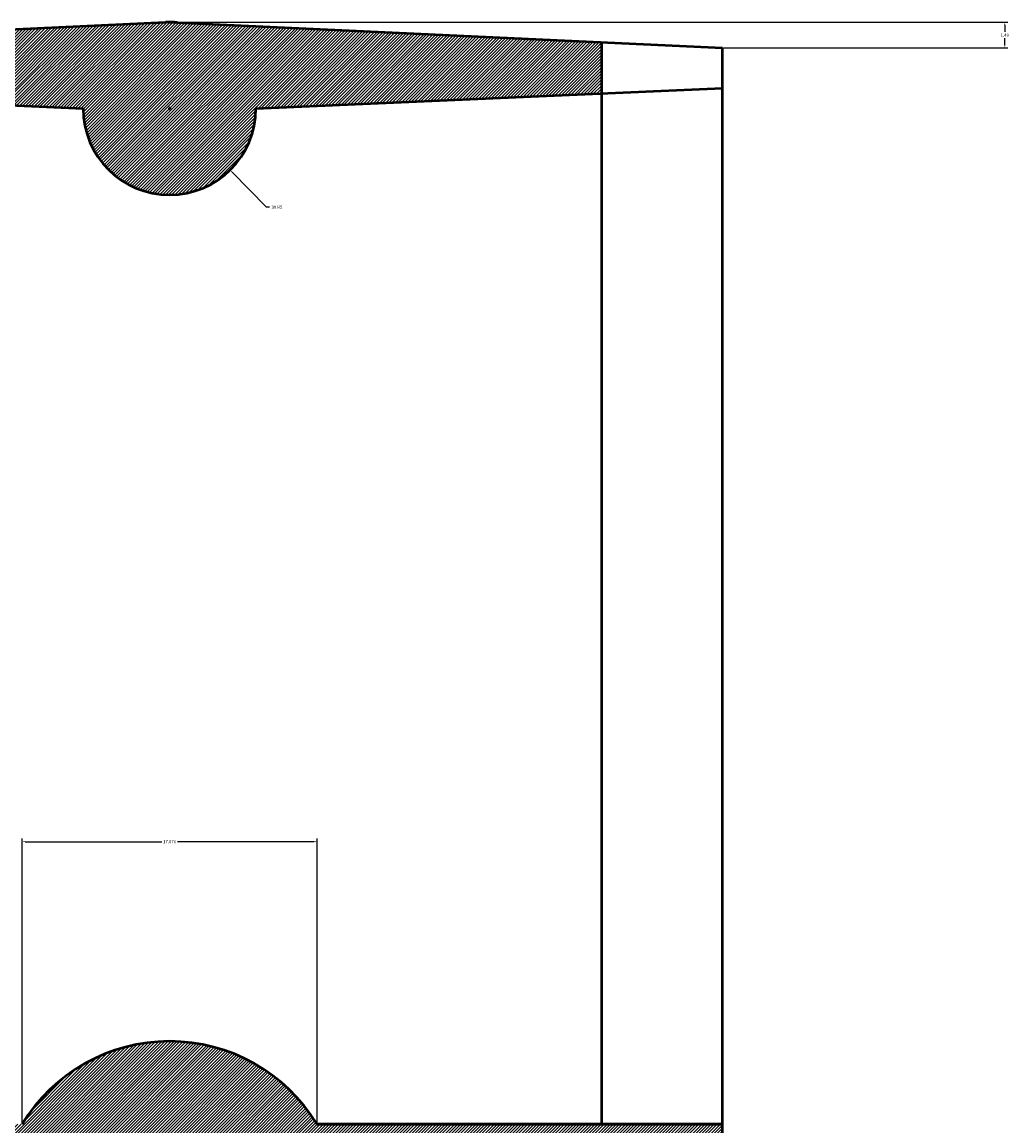
# Model space of a CAD drawing. Units: inches. Extents: x -99 to 284, y -92 to 134.
# Tile 16 of 16: x 227 to 284, y 39 to 103. Entities that reach past the tile are written whole.
import ezdxf

# ---------------------------------------------------------------- set-up
doc = ezdxf.new("R2010")
doc.units = ezdxf.units.IN
doc.header["$MEASUREMENT"] = 0
for name, color, linetype, lineweight in [('M-DIMS', 2, 'Continuous', 18), ('M-HATC', 8, 'Continuous', 18), ('M-OUTL', 7, 'Continuous', 50)]:
    doc.layers.add(name, color=color, linetype=linetype, lineweight=lineweight)
doc.styles.get("Standard").update_dxf_attribs({"font": 'arial.ttf'})
doc.dimstyles.get("Standard").update_dxf_attribs({"dimtxt": 0.18, "dimasz": 0.18, "dimexe": 0.18, "dimexo": 0.0625, "dimgap": 0.09, "dimtad": 0, "dimtih": 1, "dimtoh": 1, "dimdec": 4, "dimzin": 0, "dimdsep": 46, "dimtxsty": 'Standard', "dimcen": 0.09, "dimadec": 0, "dimazin": 0, "dimtfac": 1, "dimtdec": 4, "dimtofl": 0, "dimtmove": 0, "dimatfit": 3, "dimfxl": 1, "dimtolj": 1, "dimtzin": 0, "dimarcsym": 0})

# ---------------------------------------------------------------- blocks, each defined once
blk = doc.blocks.new('*D6')
at = {"layer": 'Defpoints', "color": 0, "transparency": 16777216}
for p in [(244.029, 55.296), (226.953, 38.946), (244.029, 38.946)]:
    blk.add_point(p, dxfattribs=at)
at = {"layer": 'M-DIMS', "color": 0, "lineweight": -2, "transparency": 16777216}
for p, q in [((226.953, 39.008), (226.953, 55.476)), ((227.133, 55.296), (235.036, 55.296)), ((243.849, 55.296), (235.946, 55.296)), ((244.029, 39.008), (244.029, 55.476))]:
    blk.add_line(p, q, dxfattribs=at)
at = {"layer": 'M-DIMS', "color": 0, "transparency": 16777216}
for points in [[(227.133, 55.326), (227.133, 55.266), (226.953, 55.296)], [(243.849, 55.326), (243.849, 55.266), (244.029, 55.296)]]:
    blk.add_solid(points, dxfattribs=at)
at = {"layer": 'M-DIMS', "color": 0, "transparency": 16777216, "insert": (235.491, 55.296), "char_height": 0.18, "attachment_point": 5}
blk.add_mtext('\\A1;17.076', dxfattribs=at)
blk = doc.blocks.new('*D11')
at = {"layer": 'Defpoints', "color": 0, "transparency": 16777216}
for p in [(235.608, 102.738), (283.841, 102.738), (267.491, 101.245)]:
    blk.add_point(p, dxfattribs=at)
at = {"layer": 'M-DIMS', "color": 0, "lineweight": -2, "transparency": 16777216}
for p, q in [((235.67, 102.738), (284.021, 102.738)), ((283.841, 102.558), (283.841, 102.173)), ((283.841, 101.425), (283.841, 101.81)), ((267.554, 101.245), (284.021, 101.245))]:
    blk.add_line(p, q, dxfattribs=at)
at = {"layer": 'M-DIMS', "color": 0, "transparency": 16777216}
for points in [[(283.811, 102.558), (283.871, 102.558), (283.841, 102.738)], [(283.811, 101.425), (283.871, 101.425), (283.841, 101.245)]]:
    blk.add_solid(points, dxfattribs=at)
at = {"layer": 'M-DIMS', "color": 0, "transparency": 16777216, "insert": (283.841, 101.992), "char_height": 0.18, "attachment_point": 5}
blk.add_mtext('\\A1;1.49', dxfattribs=at)
blk = doc.blocks.new('*D23')
at = {"layer": 'Defpoints', "color": 0, "transparency": 16777216}
for p in [(235.491, 97.74), (238.996, 94.174)]:
    blk.add_point(p, dxfattribs=at)
at = {"layer": 'M-DIMS', "color": 0, "lineweight": -2, "transparency": 16777216}
for p, q in [((235.491, 97.65), (235.491, 97.83)), ((235.401, 97.74), (235.581, 97.74)), ((241.099, 92.034), (239.122, 94.045)), ((241.279, 92.034), (241.099, 92.034))]:
    blk.add_line(p, q, dxfattribs=at)
at = {"layer": 'M-DIMS', "color": 0, "transparency": 16777216}
blk.add_solid([(239.144, 94.066), (239.101, 94.024), (238.996, 94.174)], dxfattribs=at)
at = {"layer": 'M-DIMS', "color": 0, "transparency": 16777216, "insert": (241.708, 92.034), "char_height": 0.18, "attachment_point": 5}
blk.add_mtext('\\A1;3X R5', dxfattribs=at)

msp = doc.modelspace()

# ---------------------------------------------------------------- hatches: boundary and pattern name
at = {"layer": 'M-HATC'}
h = msp.add_hatch(dxfattribs=at)
h.set_pattern_fill('ANSI31', color=256)
h.set_pattern_definition([(45, (-295.18303, 0), (-0.088388348, 0.088388348), [])])
h.paths.add_polyline_path([(235.9574, 102.7178), (260.4913, 101.5718), (260.4913, 98.6088), (240.4913, 97.7396, -1), (230.4913, 97.7396), (210.4913, 98.6088), (210.4913, 101.573), (235.4326, 102.7424), (235.4913, 102.7396, -0.0233428)])
h.paths.add_polyline_path([(226.9535, 38.946), (203.4913, 38.946), (203.4913, 30.5521), (267.4913, 30.5521), (267.4913, 38.946), (244.0291, 38.946, 0.5614625)])
h.paths.add_polyline_path([(267.4913, 30.5521), (203.4913, 30.5521), (203.4913, 28.5521), (267.4913, 28.5521)])
h.paths.add_polyline_path([(244.0291, -11.4667), (267.4913, -11.4667), (267.4913, -0.9688), (203.4913, -0.9688), (203.4913, -11.4667), (226.9535, -11.4667), (226.9535, -60.8393, -0.294228), (221.0875, -69.9448), (249.6222, -69.8159, -0.2860474), (244.0291, -60.8393)])
h.paths.add_polyline_path([(267.4913, -71.4338), (253.5949, -70.8299, -0.1036016), (249.6222, -69.8159), (221.0875, -69.9448, -0.095981), (217.3877, -70.8299), (203.4913, -71.4338), (203.4913, -73.7656), (235.2571, -75.2549, 0.0117126), (235.4913, -75.2604), (267.4913, -73.7656)])

# ---------------------------------------------------------------- linework, layer by layer
at = {"layer": 'M-OUTL'}
for p, q in [((203.4913, 101.2449), (235.2571, 102.7341)), ((235.4913, 102.7396), (267.4913, 101.2449)), ((260.4913, 101.5718), (260.4913, 38.946)), ((267.4913, 13.7396), (267.4913, 101.2449)), ((203.4913, 98.913), (230.4913, 97.7396)), ((240.4913, 97.7396), (267.4913, 98.913)), ((244.0291, 38.946), (267.4913, 38.946)), ((267.4913, 38.946), (244.0291, 38.946))]:
    msp.add_line(p, q, dxfattribs=at)
for centre, radius, start, end in [((235.4913, 97.7396), 5, 84.651198, 92.684213), ((235.4913, 97.7396), 5, 180, 0), ((235.4913, 33.7396), 10, 31.374848, 148.625152)]:
    msp.add_arc(centre, radius, start, end, dxfattribs=at)

# ---------------------------------------------------------------- dimensions: what is measured, and where the dimension line sits
at = {"layer": 'M-DIMS'}
dim = msp.add_linear_dim(base=(283.8413, 102.7383), p1=(267.4913, 101.2449), p2=(235.6075, 102.7383), angle=90, dimstyle='Standard', override={"dimdec": 2, "dimlfac": 1, "dimrnd": 0, "dimzin": 0, "dimdsep": 46, "dimlunit": 2}, dxfattribs=at)
dim.commit()
dim.dimension.update_dxf_attribs({"geometry": '*D11', "text_midpoint": (283.8413, 101.9916)})
dim = msp.add_radius_dim(center=(235.4913, 97.7396), mpoint=(238.9962, 94.1737), text='3X <>', dimstyle='Standard', override={"dimdec": 0, "dimlfac": 1, "dimrnd": 0, "dimzin": 0, "dimdsep": 46, "dimlunit": 2}, dxfattribs=at)
dim.commit()
dim.dimension.update_dxf_attribs({"geometry": '*D23', "text_midpoint": (241.7082, 92.0342), "dimtype": 164})
dim = msp.add_linear_dim(base=(244.0291, 55.296), p1=(226.9535, 38.946), p2=(244.0291, 38.946), dimstyle='Standard', override={"dimdec": 3, "dimlfac": 1, "dimrnd": 0, "dimzin": 0, "dimdsep": 46, "dimlunit": 2}, dxfattribs=at)
dim.commit()
dim.dimension.update_dxf_attribs({"geometry": '*D6', "text_midpoint": (235.4913, 55.296)})

doc.saveas('drawing.dxf')
